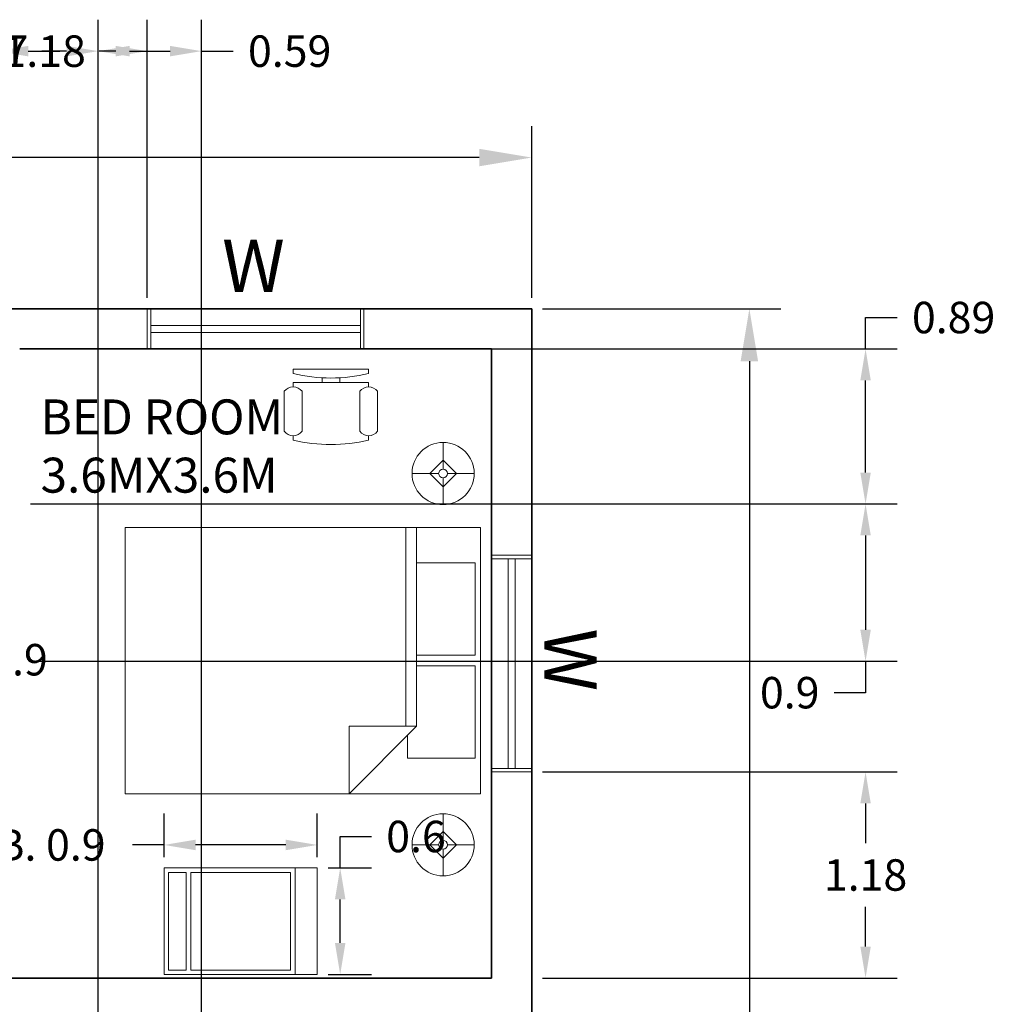
# Model space of a CAD drawing. Units: metres. Extents: x 40.9 to 56.1, y -1.4 to 24.2.
# Tile 7 of 7: x 49.6 to 55.2, y 18.6 to 24.2. Entities that reach past the tile are written whole.
import ezdxf

# ---------------------------------------------------------------- set-up
doc = ezdxf.new("R2010")
doc.units = ezdxf.units.M
doc.header["$MEASUREMENT"] = 0
for name, color, linetype, lineweight in [('A-ANNO-DIMS', 2, 'Continuous', 18), ('A-ANNO-TEXT', 7, 'Continuous', 18), ('A-AREA-IDEN', 7, 'Continuous', 18), ('A-FLOR-CASE', 9, 'Continuous', 18), ('A-FURN', 8, 'Continuous', 18), ('A-GLAZ', 4, 'Continuous', 18), ('A-WALL', 7, 'Continuous', 35)]:
    doc.layers.add(name, color=color, linetype=linetype, lineweight=lineweight)
doc.styles.get("Standard").update_dxf_attribs({"font": 'arial.ttf'})
doc.dimstyles.get("Standard").update_dxf_attribs({"dimtxt": 0.18, "dimasz": 0.18, "dimexe": 0.18, "dimexo": 0.0625, "dimgap": 0.09, "dimtad": 0, "dimtih": 1, "dimtoh": 1, "dimdec": 1, "dimzin": 0, "dimdsep": 46, "dimtxsty": 'Standard', "dimcen": 0.09, "dimadec": 0, "dimazin": 0, "dimtfac": 1, "dimtdec": 1, "dimtofl": 0, "dimtmove": 0, "dimatfit": 3, "dimfxl": 1, "dimtolj": 1, "dimtzin": 0, "dimarcsym": 0})

# ---------------------------------------------------------------- blocks, each defined once
blk = doc.blocks.new('Bed - Queen')
for p, q in [((0, -80.00003), (0, 0)), ((0, 0), (59.99999, 0)), ((59.99999, 0), (59.99999, -80.00003)), ((7.99999, -1.2), (28.79998, -1.2)), ((7.99999, -14.4), (7.99999, -1.2)), ((28.79998, -1.2), (28.79998, -14.4)), ((31.19999, -1.2), (51.99999, -1.2)), ((31.19999, -14.4), (31.19999, -1.2)), ((51.99999, -1.2), (51.99999, -16.4)), ((0, -14.4), (44.8, -14.4)), ((59.99999, -29.6), (44.8, -14.4)), ((44.8, -14.4), (44.8, -29.6)), ((44.8, -16.8), (0, -16.8)), ((51.99999, -16.4), (46.79936, -16.4)), ((44.8, -29.6), (59.99999, -29.6)), ((59.99999, -80.00003), (0, -80.00003))]:
    blk.add_line(p, q)
blk = doc.blocks.new('Lamp - Table')
for p, q in [((0, 7), (0, 1)), ((0, 3), (-3, 0)), ((3, 0), (0, 3)), ((-1, 0), (-7, 0)), ((-3, 0), (0, -3)), ((0, -3), (3, 0)), ((1, 0), (7, 0)), ((0, -1), (0, -7))]:
    blk.add_line(p, q)
for radius in [7, 1]:
    blk.add_circle((0, 0), radius)
blk = doc.blocks.new('Chair - Desk')
for p, q in [((-8.5, 0), (-8.5, -1)), ((-8.5, 0), (8.5, 0)), ((8.5, 0), (8.5, -1)), ((-2, -3), (-2, -1.9355)), ((2, -1.9576), (2, -3)), ((-8.5, -3), (-8.5, -4)), ((-8.5, -3), (8.5, -3)), ((8.5, -3), (8.5, -4)), ((-10.5, -5), (-10.5, -14)), ((-6.5, -14), (-6.5, -5)), ((6.5, -5), (6.5, -14)), ((10.5, -14), (10.5, -5)), ((-8.5, -15), (-8.5, -16)), ((8.5, -15), (8.5, -16))]:
    blk.add_line(p, q)
for centre, radius, start, end in [((0, 34.625), 36.625, 256.5803, 283.4197), ((-8.5, -6.5), 2.5, 36.8699, 143.1301), ((8.5, -6.5), 2.5, 36.8699, 143.1301), ((-8.5, -12.5), 2.5, 216.8699, 323.1301), ((8.5, -12.5), 2.5, 216.8699, 323.1301), ((0, 19.625), 36.625, 256.5803, 283.4197)]:
    blk.add_arc(centre, radius, start, end)
blk = doc.blocks.new('Base Cabinet 1 Door - 24 in front')
for p, q in [((0, 0), (0, 34.5)), ((0, 34.5), (24, 34.5)), ((1, 29.5), (1, 33.5)), ((1, 33.5), (23, 33.5)), ((23, 33.5), (23, 29.5)), ((24, 34.5), (24, 0)), ((1, 29.5), (23, 29.5)), ((23, 28.5), (1, 28.5)), ((1, 6), (1, 28.5)), ((23, 28.5), (23, 6)), ((0, 5), (24, 5)), ((23, 6), (1, 6)), ((24, 0), (0, 0))]:
    blk.add_line(p, q)
blk = doc.blocks.new('*D45')
at = {"layer": 'A-ANNO-DIMS', "color": 0, "lineweight": -2, "transparency": 16777216}
for p, q in [((45.2552, 22.6498), (45.2552, 23.6329)), ((52.5152, 22.6498), (52.5152, 23.6329)), ((45.5552, 23.4529), (48.5233, 23.4529)), ((52.2152, 23.4529), (49.2471, 23.4529))]:
    blk.add_line(p, q, dxfattribs=at)
at = {"layer": 'A-ANNO-DIMS', "color": 0, "transparency": 16777216}
for points in [[(45.5552, 23.5029), (45.5552, 23.4029), (45.2552, 23.4529)], [(52.2152, 23.5029), (52.2152, 23.4029), (52.5152, 23.4529)]]:
    blk.add_solid(points, dxfattribs=at)
at = {"layer": 'Defpoints', "color": 0, "transparency": 16777216}
for p in [(52.5152, 23.4529), (45.2552, 22.5873), (52.5152, 22.5873)]:
    blk.add_point(p, dxfattribs=at)
at = {"layer": 'A-ANNO-DIMS', "color": 0, "transparency": 16777216, "insert": (48.8852, 23.4529), "char_height": 0.3, "attachment_point": 5}
blk.add_mtext('\\A1;7.3', dxfattribs=at)
blk = doc.blocks.new('*D46')
at = {"layer": 'A-ANNO-DIMS', "color": 0, "lineweight": -2, "transparency": 16777216}
for p, q in [((52.5777, 22.5873), (53.9408, 22.5873)), ((53.7608, 22.2873), (53.7608, 15.8755)), ((53.7608, 8.9773), (53.7608, 15.389)), ((52.5777, 8.6773), (53.9408, 8.6773))]:
    blk.add_line(p, q, dxfattribs=at)
at = {"layer": 'A-ANNO-DIMS', "color": 0, "transparency": 16777216}
for points in [[(53.7108, 22.2873), (53.8108, 22.2873), (53.7608, 22.5873)], [(53.7108, 8.9773), (53.8108, 8.9773), (53.7608, 8.6773)]]:
    blk.add_solid(points, dxfattribs=at)
at = {"layer": 'Defpoints', "color": 0, "transparency": 16777216}
for p in [(52.5152, 22.5873), (52.5152, 8.6773), (53.7608, 8.6773)]:
    blk.add_point(p, dxfattribs=at)
at = {"layer": 'A-ANNO-DIMS', "color": 0, "transparency": 16777216, "insert": (53.7608, 15.6323), "char_height": 0.3, "attachment_point": 5}
blk.add_mtext('\\A1;13.9', dxfattribs=at)
blk = doc.blocks.new('WIN-1200-PLAN')
for p, q in [((-0.0002, 0.0003), (-0.0002, 0.2303)), ((0.0198, 0.0003), (0.0198, 0.2303)), ((1.2198, 0.0003), (1.2198, 0.2303)), ((1.2398, 0.0003), (1.2398, 0.2303)), ((0.0198, 0.1353), (1.2198, 0.1353)), ((0.0198, 0.0953), (1.2198, 0.0953))]:
    blk.add_line(p, q)
blk = doc.blocks.new('*D94')
at = {"layer": 'A-ANNO-DIMS', "color": 0, "lineweight": -2, "transparency": 16777216}
for p, q in [((48.227, 20.7453), (48.227, 20.3992)), ((49.1414, 20.7453), (49.1414, 20.3992)), ((48.407, 20.5792), (48.9614, 20.5792)), ((49.1414, 20.5792), (49.3214, 20.5792))]:
    blk.add_line(p, q, dxfattribs=at)
at = {"layer": 'A-ANNO-DIMS', "color": 0, "transparency": 16777216}
for points in [[(48.407, 20.6092), (48.407, 20.5492), (48.227, 20.5792)], [(48.9614, 20.6092), (48.9614, 20.5492), (49.1414, 20.5792)]]:
    blk.add_solid(points, dxfattribs=at)
at = {"layer": 'Defpoints', "color": 0, "transparency": 16777216}
for p in [(48.227, 20.8078), (49.1414, 20.8078), (49.1414, 20.5792)]:
    blk.add_point(p, dxfattribs=at)
at = {"layer": 'A-ANNO-DIMS', "color": 0, "transparency": 16777216, "insert": (49.5754, 20.5792), "char_height": 0.18, "attachment_point": 5}
blk.add_mtext('\\A1;0.9', dxfattribs=at)
blk = doc.blocks.new('*D111')
at = {"layer": 'A-ANNO-DIMS', "color": 0, "lineweight": -2, "transparency": 16777216}
for p, q in [((50.4115, 19.4502), (50.4115, 19.6992)), ((51.2878, 19.4502), (51.2878, 19.6992)), ((50.4115, 19.5192), (50.2315, 19.5192)), ((51.1078, 19.5192), (50.5915, 19.5192))]:
    blk.add_line(p, q, dxfattribs=at)
at = {"layer": 'A-ANNO-DIMS', "color": 0, "transparency": 16777216}
for points in [[(50.5915, 19.5492), (50.5915, 19.4892), (50.4115, 19.5192)], [(51.1078, 19.5492), (51.1078, 19.4892), (51.2878, 19.5192)]]:
    blk.add_solid(points, dxfattribs=at)
at = {"layer": 'Defpoints', "color": 0, "transparency": 16777216}
for p in [(50.4115, 19.5192), (50.4115, 19.3877), (51.2878, 19.3877)]:
    blk.add_point(p, dxfattribs=at)
at = {"layer": 'A-ANNO-DIMS', "color": 0, "transparency": 16777216, "insert": (49.2827, 19.5192), "char_height": 0.18, "attachment_point": 5}
blk.add_mtext('\\A1;BASE CAB. 0.9', dxfattribs=at)
blk = doc.blocks.new('*D112')
at = {"layer": 'A-ANNO-DIMS', "color": 0, "lineweight": -2, "transparency": 16777216}
for p, q in [((51.4193, 19.3877), (51.4193, 19.5677)), ((51.4193, 19.5677), (51.5993, 19.5677)), ((51.3503, 19.3877), (51.5993, 19.3877)), ((51.4193, 18.9581), (51.4193, 19.2077)), ((51.3503, 18.7781), (51.5993, 18.7781))]:
    blk.add_line(p, q, dxfattribs=at)
at = {"layer": 'A-ANNO-DIMS', "color": 0, "transparency": 16777216}
for points in [[(51.3893, 19.2077), (51.4493, 19.2077), (51.4193, 19.3877)], [(51.3893, 18.9581), (51.4493, 18.9581), (51.4193, 18.7781)]]:
    blk.add_solid(points, dxfattribs=at)
at = {"layer": 'Defpoints', "color": 0, "transparency": 16777216}
for p in [(51.2878, 19.3877), (51.4193, 19.3877), (51.2878, 18.7781)]:
    blk.add_point(p, dxfattribs=at)
at = {"layer": 'A-ANNO-DIMS', "color": 0, "transparency": 16777216, "insert": (51.8531, 19.5677), "char_height": 0.18, "attachment_point": 5}
blk.add_mtext('\\A1;0.6', dxfattribs=at)
blk = doc.blocks.new('*D136')
at = {"layer": 'A-ANNO-DIMS', "color": 0, "lineweight": -2, "transparency": 16777216}
for p, q in [((48.7602, 14.8764), (48.7602, 24.2418)), ((49.4546, 14.8764), (49.4546, 24.2418)), ((48.5802, 24.0618), (48.4002, 24.0618)), ((49.6346, 24.0618), (49.8146, 24.0618))]:
    blk.add_line(p, q, dxfattribs=at)
at = {"layer": 'A-ANNO-DIMS', "color": 0, "transparency": 16777216}
for points in [[(48.5802, 24.0918), (48.5802, 24.0318), (48.7602, 24.0618)], [(49.6346, 24.0918), (49.6346, 24.0318), (49.4546, 24.0618)]]:
    blk.add_solid(points, dxfattribs=at)
at = {"layer": 'Defpoints', "color": 0, "transparency": 16777216}
for p in [(49.4546, 24.0618), (48.7602, 14.8139), (49.4546, 14.8139)]:
    blk.add_point(p, dxfattribs=at)
at = {"layer": 'A-ANNO-DIMS', "color": 0, "transparency": 16777216, "insert": (49.1074, 24.0618), "char_height": 0.18, "attachment_point": 5}
blk.add_mtext('\\A1;0.69', dxfattribs=at)
blk = doc.blocks.new('*D142')
at = {"layer": 'A-ANNO-DIMS', "color": 0, "lineweight": -2, "transparency": 16777216}
for p, q in [((52.5777, 19.9373), (54.6058, 19.9373)), ((54.4258, 19.7573), (54.4258, 19.5292)), ((54.4258, 18.9373), (54.4258, 19.1653)), ((52.5777, 18.7573), (54.6058, 18.7573))]:
    blk.add_line(p, q, dxfattribs=at)
at = {"layer": 'A-ANNO-DIMS', "color": 0, "transparency": 16777216}
for points in [[(54.3958, 19.7573), (54.4558, 19.7573), (54.4258, 19.9373)], [(54.3958, 18.9373), (54.4558, 18.9373), (54.4258, 18.7573)]]:
    blk.add_solid(points, dxfattribs=at)
at = {"layer": 'Defpoints', "color": 0, "transparency": 16777216}
for p in [(52.5152, 19.9373), (54.4258, 19.9373), (52.5152, 18.7573)]:
    blk.add_point(p, dxfattribs=at)
at = {"layer": 'A-ANNO-DIMS', "color": 0, "transparency": 16777216, "insert": (54.4258, 19.3473), "char_height": 0.18, "attachment_point": 5}
blk.add_mtext('\\A1;1.18', dxfattribs=at)
blk = doc.blocks.new('*D147')
at = {"layer": 'A-ANNO-DIMS', "color": 0, "lineweight": -2, "transparency": 16777216}
for p, q in [((49.1352, 22.6498), (49.1352, 24.2418)), ((50.3152, 22.6498), (50.3152, 24.2418)), ((49.3152, 24.0618), (49.4097, 24.0618)), ((50.1352, 24.0618), (50.0407, 24.0618))]:
    blk.add_line(p, q, dxfattribs=at)
at = {"layer": 'A-ANNO-DIMS', "color": 0, "transparency": 16777216}
for points in [[(49.3152, 24.0918), (49.3152, 24.0318), (49.1352, 24.0618)], [(50.1352, 24.0918), (50.1352, 24.0318), (50.3152, 24.0618)]]:
    blk.add_solid(points, dxfattribs=at)
at = {"layer": 'Defpoints', "color": 0, "transparency": 16777216}
for p in [(50.3152, 24.0618), (49.1352, 22.5873), (50.3152, 22.5873)]:
    blk.add_point(p, dxfattribs=at)
at = {"layer": 'A-ANNO-DIMS', "color": 0, "transparency": 16777216, "insert": (49.7252, 24.0618), "char_height": 0.18, "attachment_point": 5}
blk.add_mtext('\\A1;1.18', dxfattribs=at)
blk = doc.blocks.new('*D150')
at = {"layer": 'A-ANNO-DIMS', "color": 0, "lineweight": -2, "transparency": 16777216}
for p, q in [((50.034, 14.9198), (50.034, 24.2418)), ((50.6262, 14.6143), (50.6262, 24.2418)), ((50.214, 24.0618), (50.4462, 24.0618)), ((50.6262, 24.0618), (50.8062, 24.0618))]:
    blk.add_line(p, q, dxfattribs=at)
at = {"layer": 'A-ANNO-DIMS', "color": 0, "transparency": 16777216}
for points in [[(50.214, 24.0918), (50.214, 24.0318), (50.034, 24.0618)], [(50.4462, 24.0918), (50.4462, 24.0318), (50.6262, 24.0618)]]:
    blk.add_solid(points, dxfattribs=at)
at = {"layer": 'Defpoints', "color": 0, "transparency": 16777216}
for p in [(50.6262, 24.0618), (50.034, 14.8573), (50.6262, 14.5518)]:
    blk.add_point(p, dxfattribs=at)
at = {"layer": 'A-ANNO-DIMS', "color": 0, "transparency": 16777216, "insert": (51.1301, 24.0618), "char_height": 0.18, "attachment_point": 5}
blk.add_mtext('\\A1;0.59', dxfattribs=at)
blk = doc.blocks.new('*D154')
at = {"layer": 'A-ANNO-DIMS', "color": 0, "lineweight": -2, "transparency": 16777216}
for p, q in [((48.7602, 13.2198), (48.7602, 24.2418)), ((50.034, 13.2198), (50.034, 24.2418)), ((48.9402, 24.0618), (49.0818, 24.0618)), ((49.854, 24.0618), (49.7124, 24.0618))]:
    blk.add_line(p, q, dxfattribs=at)
at = {"layer": 'A-ANNO-DIMS', "color": 0, "transparency": 16777216}
for points in [[(48.9402, 24.0918), (48.9402, 24.0318), (48.7602, 24.0618)], [(49.854, 24.0918), (49.854, 24.0318), (50.034, 24.0618)]]:
    blk.add_solid(points, dxfattribs=at)
at = {"layer": 'Defpoints', "color": 0, "transparency": 16777216}
for p in [(50.034, 24.0618), (48.7602, 13.1573), (50.034, 13.1573)]:
    blk.add_point(p, dxfattribs=at)
at = {"layer": 'A-ANNO-DIMS', "color": 0, "transparency": 16777216, "insert": (49.3971, 24.0618), "char_height": 0.18, "attachment_point": 5}
blk.add_mtext('\\A1;1.27', dxfattribs=at)
blk = doc.blocks.new('*D157')
at = {"layer": 'A-ANNO-DIMS', "color": 0, "lineweight": -2, "transparency": 16777216}
for p, q in [((49.6477, 21.4705), (54.6058, 21.4705)), ((54.4258, 21.2905), (54.4258, 20.7505)), ((49.6477, 20.5705), (54.6058, 20.5705)), ((54.4258, 20.5705), (54.4258, 20.3905)), ((54.4258, 20.3905), (54.2458, 20.3905))]:
    blk.add_line(p, q, dxfattribs=at)
at = {"layer": 'A-ANNO-DIMS', "color": 0, "transparency": 16777216}
for points in [[(54.3958, 21.2905), (54.4558, 21.2905), (54.4258, 21.4705)], [(54.3958, 20.7505), (54.4558, 20.7505), (54.4258, 20.5705)]]:
    blk.add_solid(points, dxfattribs=at)
at = {"layer": 'Defpoints', "color": 0, "transparency": 16777216}
for p in [(49.5852, 21.4705), (49.5852, 20.5705), (54.4258, 20.5705)]:
    blk.add_point(p, dxfattribs=at)
at = {"layer": 'A-ANNO-DIMS', "color": 0, "transparency": 16777216, "insert": (53.9918, 20.3905), "char_height": 0.18, "attachment_point": 5}
blk.add_mtext('\\A1;0.9', dxfattribs=at)
blk = doc.blocks.new('*D158')
at = {"layer": 'A-ANNO-DIMS', "color": 0, "lineweight": -2, "transparency": 16777216}
for p, q in [((54.4258, 22.3573), (54.4258, 22.5373)), ((54.4258, 22.5373), (54.6058, 22.5373)), ((49.6477, 22.3573), (54.6058, 22.3573)), ((54.4258, 21.6505), (54.4258, 22.1773)), ((49.6477, 21.4705), (54.6058, 21.4705))]:
    blk.add_line(p, q, dxfattribs=at)
at = {"layer": 'A-ANNO-DIMS', "color": 0, "transparency": 16777216}
for points in [[(54.3958, 22.1773), (54.4558, 22.1773), (54.4258, 22.3573)], [(54.3958, 21.6505), (54.4558, 21.6505), (54.4258, 21.4705)]]:
    blk.add_solid(points, dxfattribs=at)
at = {"layer": 'Defpoints', "color": 0, "transparency": 16777216}
for p in [(49.5852, 22.3573), (54.4258, 22.3573), (49.5852, 21.4705)]:
    blk.add_point(p, dxfattribs=at)
at = {"layer": 'A-ANNO-DIMS', "color": 0, "transparency": 16777216, "insert": (54.9298, 22.5373), "char_height": 0.18, "attachment_point": 5}
blk.add_mtext('\\A1;0.89', dxfattribs=at)

msp = doc.modelspace()

# ---------------------------------------------------------------- linework, layer by layer
at = {"layer": 'A-WALL'}
for p, q in [((48.6852, 22.5873), (52.5152, 22.5873)), ((52.5152, 22.5873), (52.5152, 18.7573)), ((49.5852, 22.3573), (52.2852, 22.3573)), ((52.2852, 22.3573), (52.2852, 18.7573)), ((52.2852, 18.7573), (49.5085, 18.7573)), ((52.5152, 18.7573), (52.5152, 13.1573))]:
    msp.add_line(p, q, dxfattribs=at)

# ---------------------------------------------------------------- block references
at = {"layer": 'A-FLOR-CASE', "xscale": 0.0254, "yscale": 0.0254, "zscale": 0.0254, "rotation": 90}
msp.add_blockref('Base Cabinet 1 Door - 24 in front', (51.2878, 18.7781), dxfattribs=at)
at = {"layer": 'A-FURN', "xscale": 0.0254, "yscale": 0.0254, "zscale": 0.0254}
for name, p in [('Chair - Desk', (51.3662, 22.2421)), ('Lamp - Table', (52.0082, 21.6449)), ('Lamp - Table', (52.0082, 19.5201))]:
    msp.add_blockref(name, p, dxfattribs=at)
at = {"layer": 'A-FURN', "xscale": 0.0254, "yscale": 0.0254, "zscale": 0.0254, "rotation": 270}
msp.add_blockref('Bed - Queen', (52.2217, 21.3365), dxfattribs=at)
at = {"layer": 'A-GLAZ'}
for p, rotation in [((51.5551, 22.5875), 180), ((52.5155, 19.9374), 89.99999999999947)]:
    msp.add_blockref('WIN-1200-PLAN', p, dxfattribs=dict(at, rotation=rotation))

# ---------------------------------------------------------------- texts
at = {"layer": 'A-ANNO-TEXT'}
msp.add_text('W', height=0.3, dxfattribs=at).set_placement((50.7434, 22.6829))
msp.add_text('W', height=0.3, rotation=270, dxfattribs=at).set_placement((52.5874, 20.7582))
at = {"layer": 'A-AREA-IDEN', "insert": (49.7048, 22.0687), "char_height": 0.2, "attachment_point": 1}
msp.add_mtext_dynamic_manual_height_columns('BED ROOM\\P3.6MX3.6M', width=2.030673, gutter_width=1, heights=[0], dxfattribs=at)

# ---------------------------------------------------------------- dimensions: what is measured, and where the dimension line sits
at = {"layer": 'A-ANNO-DIMS'}
for base, p1, p2, override, picture, middle in [((49.4546, 24.0618), (48.7602, 14.8139), (49.4546, 14.8139), {"dimdec": 2, "dimlfac": 1, "dimrnd": 0, "dimzin": 0, "dimdsep": 46, "dimlunit": 2}, '*D136', (49.1074, 24.0618)), ((50.034, 24.0618), (48.7602, 13.1573), (50.034, 13.1573), {"dimdec": 2, "dimlfac": 1, "dimrnd": 0, "dimzin": 0, "dimdsep": 46, "dimlunit": 2}, '*D154', (49.3971, 24.0618)), ((50.3152, 24.0618), (49.1352, 22.5873), (50.3152, 22.5873), {"dimdec": 2, "dimlfac": 1, "dimrnd": 0, "dimzin": 0, "dimdsep": 46, "dimlunit": 2}, '*D147', (49.7252, 24.0618)), ((50.6262, 24.0618), (50.034, 14.8573), (50.6262, 14.5518), {"dimdec": 2, "dimlfac": 1, "dimrnd": 0, "dimzin": 0, "dimdsep": 46, "dimlunit": 2}, '*D150', (51.1301, 24.0618)), ((52.5152, 23.4529), (45.2552, 22.5873), (52.5152, 22.5873), {"dimtxt": 0.3, "dimasz": 0.3, "dimclrd": 0, "dimclre": 0, "dimclrt": 0}, '*D45', (48.8852, 23.4529)), ((49.1414, 20.5792), (48.227, 20.8078), (49.1414, 20.8078), {"dimdec": 1, "dimlfac": 1, "dimrnd": 0, "dimzin": 0, "dimdsep": 46, "dimlunit": 2}, '*D94', (49.5754, 20.5792))]:
    dim = msp.add_linear_dim(base=base, p1=p1, p2=p2, dimstyle='Standard', override=override, dxfattribs=at)
    dim.commit()
    dim.dimension.update_dxf_attribs({"geometry": picture, "text_midpoint": middle})
for base, p1, p2, override, picture, middle in [((54.4258, 22.3573), (49.5852, 21.4705), (49.5852, 22.3573), {"dimdec": 2, "dimlfac": 1, "dimrnd": 0, "dimzin": 0, "dimdsep": 46, "dimlunit": 2}, '*D158', (54.9298, 22.5373)), ((53.7608, 8.6773), (52.5152, 22.5873), (52.5152, 8.6773), {"dimtxt": 0.3, "dimasz": 0.3, "dimclrd": 0, "dimclre": 0, "dimclrt": 0}, '*D46', (53.7608, 15.6323)), ((54.4258, 20.5705), (49.5852, 21.4705), (49.5852, 20.5705), {"dimdec": 1, "dimlfac": 1, "dimrnd": 0, "dimzin": 0, "dimdsep": 46, "dimlunit": 2}, '*D157', (53.9918, 20.3905)), ((54.4258, 19.9373), (52.5152, 18.7573), (52.5152, 19.9373), {"dimdec": 2, "dimlfac": 1, "dimrnd": 0, "dimzin": 0, "dimdsep": 46, "dimlunit": 2}, '*D142', (54.4258, 19.3473)), ((51.4193, 19.3877), (51.2878, 18.7781), (51.2878, 19.3877), {"dimdec": 1, "dimlfac": 1, "dimrnd": 0, "dimzin": 0, "dimdsep": 46, "dimlunit": 2}, '*D112', (51.8531, 19.5677))]:
    dim = msp.add_linear_dim(base=base, p1=p1, p2=p2, angle=90, dimstyle='Standard', override=override, dxfattribs=at)
    dim.commit()
    dim.dimension.update_dxf_attribs({"geometry": picture, "text_midpoint": middle})
dim = msp.add_linear_dim(base=(50.4115, 19.5192), p1=(51.2878, 19.3877), p2=(50.4115, 19.3877), angle=180, text='BASE CAB. <>', dimstyle='Standard', override={"dimdec": 1, "dimlfac": 1, "dimrnd": 0, "dimzin": 0, "dimdsep": 46, "dimlunit": 2}, dxfattribs=at)
dim.commit()
dim.dimension.update_dxf_attribs({"geometry": '*D111', "text_midpoint": (49.2827, 19.5192)})

doc.saveas('drawing.dxf')
